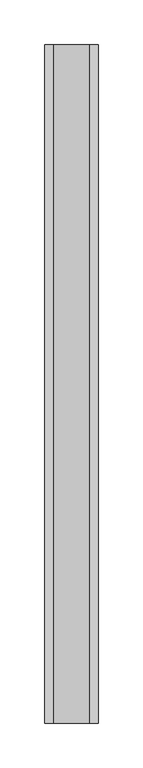
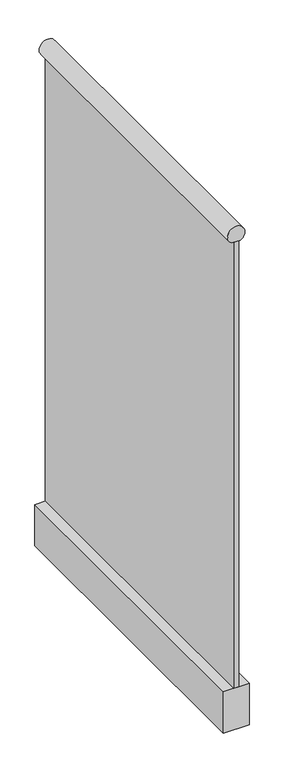
"""IFC4 building model written with IfcOpenShell, lengths in millimetres: railing geometry."""

from ifc_helpers import new_model, si_unit, point, frame, frame_2d, origin, place, context, project, spatial, polyline, circle_curve, trimmed, segment, composite_curve, outline, extrude, source, transform, mapped, element, save


def railing_ba9b8cd4(model_context):
    return source(origin(), model_context, "Body", "SweptSolid", [
        extrude(outline(composite_curve([segment(trimmed(circle_curve(frame_2d((8465.3205081, -1533.8712297)), 20.0), [point((8448.0, -1523.8712297))], [point((8448.0, -1543.8712297))], False, "CARTESIAN"), True, "CONTINUOUS"), segment(polyline([(8448.0, -1543.8712297), (8448.0, -1523.8712297)]), True, "CONTINUOUS")], self_intersect=False)), frame((0.0, -6422.0014262, 0.0), z_axis=(0.0, 1.0, 0.0), x_axis=(0.0, 0.0, 1.0)), (0.0, 0.0, 1.0), 760.0),
        extrude(outline(polyline([(-1527.8712297, -6422.0014262), (-1539.8712297, -6422.0014262), (-1539.8712297, -5662.0014262), (-1527.8712297, -5662.0014262), (-1527.8712297, -6422.0014262)])), frame((0.0, 0.0, 7350.0), z_axis=(0.0, 0.0, 1.0), x_axis=(1.0, 0.0, 0.0)), (0.0, 0.0, 1.0), 1098.0),
        extrude(outline(polyline([(-1503.8712297, -6422.0014262), (-1563.8712297, -6422.0014262), (-1563.8712297, -5662.0014262), (-1503.8712297, -5662.0014262), (-1503.8712297, -6422.0014262)])), frame((0.0, 0.0, 7248.0), z_axis=(0.0, 0.0, 1.0), x_axis=(1.0, 0.0, 0.0)), (0.0, 0.0, 1.0), 102.0),
    ])


if __name__ == "__main__":
    model = new_model("IFC4")
    model_context = context("Model", 3, world=origin())
    ifc_project = project(units=[si_unit("LENGTHUNIT", "METRE", prefix="MILLI")], contexts=[model_context])
    site = spatial("IfcSite", under=ifc_project)
    building = spatial("IfcBuilding", under=site)
    placement = place(None, origin())
    railing_shape = railing_ba9b8cd4(model_context)
    element("IfcRailing", 1, at=placement, inside=building, context=model_context, shape_type="MappedRepresentation", body=[
        mapped(railing_shape, transform((0.0, 0.0, 0.0), x_axis=(1.0, 0.0, 0.0), y_axis=(0.0, 1.0, 0.0), z_axis=(0.0, 0.0, 1.0))),
    ])
    save(model, "model.ifc")

# Revit data of these elements
# Element 1 (IfcRailing)
#   Materials on its faces: "Metal - Aluminum"
# Materials
#   "Metal - Aluminum": colour RGB 247 247 247, transparency 0, Cost = 0
